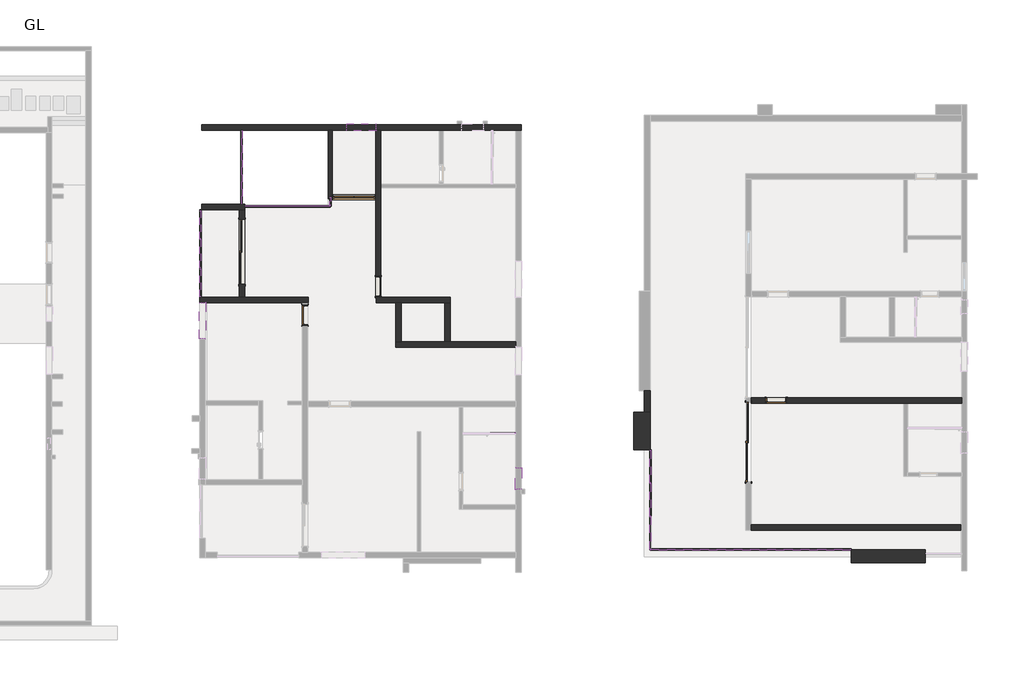
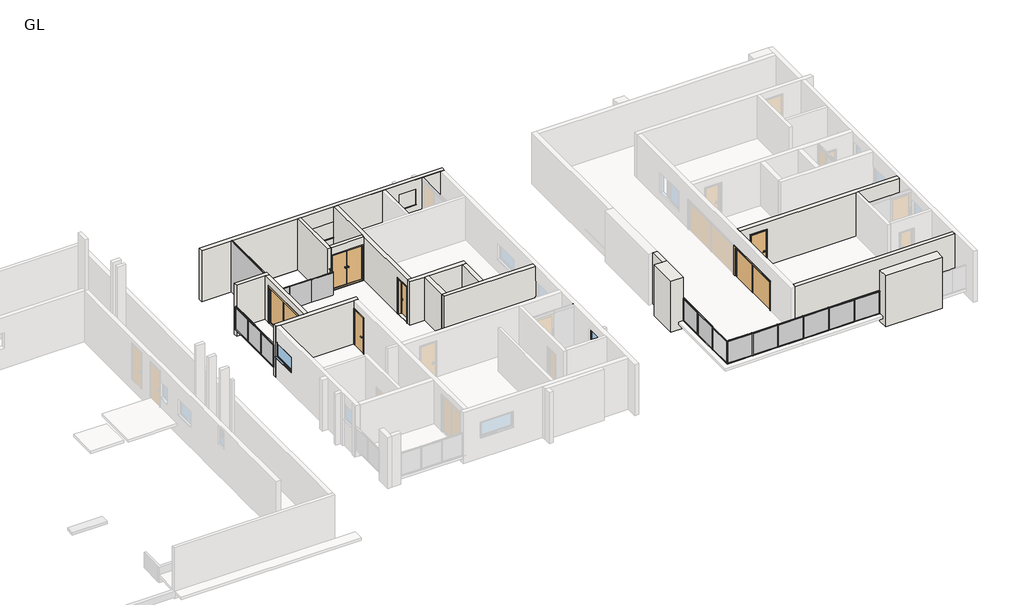
# One storey, part 3 of 6: 60 members, 17 walls, 16 plates, 6 doors, 3 windows.
# Revit data of these elements (continued)
# Elements 4, 5, 6 (IfcDoor, "Doors_IntSgl : 2'11\"") (continued)
#   Materials on its faces: "Door - Architrave", "Door - Handle", "Door - Frame/Mullion (1)", "Door - Panel"
# Elements 7, 8, 9, 10, 11, 12, 13, 14, 15, 16, 17, 18, 19, 20, 21, 22, 23, 24, 25, 26, 27, 28, 29, 30, 31, 32, 33, 34, 35, 36, 37, 38, 39, 40, 41, 42, 43, 44, 45, 46, 47, 48, 49, 50, 51, 52, 53, 54, 55, 56, 57, 58, 59, 60, 61, 62, 63, 64, 65, 66 (IfcMember, "Rectangular Mullion : 30mm_Square")
#   Phase Created = New Construction
#   Materials on its faces: "Aluminium"
# Elements 67, 68, 69, 70, 71, 72, 73, 74, 75, 76, 77, 78, 79, 80, 81, 82 (IfcPlate, "System Panel : Glazed")
#   Phase Created = New Construction
#   Materials on its faces: "Glass"
# Element 83 (IfcWall, "1'10\"")
#   Top Offset = 0' - 0"
#   Base Offset = 0' - 0"
#   wall height = 9' - 10.11024"
#   Phase Created = New Construction
#   Base Constraint = GL
#   Top Constraint = FFL
#   Materials on its faces: "Brick, Common"
# Element 84 (IfcWall, "10\"")
#   Top Offset = 0' - 0"
#   Base Offset = 0' - 0"
#   wall height = 9' - 10.11024"
#   Phase Created = New Construction
#   Base Constraint = GL
#   Top Constraint = FFL
#   Materials on its faces: "Brick, Common"
# Element 85 (IfcWall, "2'3\"")
#   Top Offset = 0' - 0"
#   Base Offset = 0' - 0"
#   wall height = 9' - 10.11024"
#   Phase Created = New Construction
#   Base Constraint = GL
#   Top Constraint = FFL
#   Materials on its faces: "Brick, Common"
# Elements 86, 87 (IfcWall, "7\" WALL")
#   Top Offset = 0' - 0"
#   Base Offset = 0' - 0"
#   wall height = 9' - 10.11024"
#   Phase Created = New Construction
#   Base Constraint = GL
#   Top Constraint = FFL
#   Materials on its faces: "Brick, Common"
# Elements 88, 89, 90, 91, 92, 93, 94, 95, 96, 97, 98, 99 (IfcWall, "9\" INNER WALL")
#   Top Offset = 0' - 0"
#   Base Offset = 0' - 0"
#   wall height = 9' - 10.11024"
#   Phase Created = New Construction
#   Base Constraint = GL
#   Top Constraint = FFL
#   Materials on its faces: "Brick, Common"
# Element 100 (IfcWindow, "Windows_Sgl_Plain : 3'")
#   Mark = "15"
#   Phase Created = New Construction
#   Materials on its faces: "Window Frame", "Glass"
# Element 101 (IfcWindow, "Windows_Sgl_Plain : 4'")
#   Mark = "11"
#   Phase Created = New Construction
#   Materials on its faces: "Window Frame", "Glass"
# Element 102 (IfcWindow, "Windows_Sgl_Plain : 5'")
#   Mark = "18"
#   Phase Created = New Construction
#   Materials on its faces: "Window Frame", "Glass"
# Materials
#   "Puerta - Panel": class "Madera", colour RGB 210 159 95, transparency 0
#   "Door - Panel": class "Wood", colour RGB 210 159 95, transparency 0, Keynote = "L20", Cost = 0
#   "Door - Frame/Mullion": class "Wood", colour RGB 212 179 113, transparency 0, Keynote = "L20", Cost = 0
#   "Door - Handle": colour RGB 0 0 0, transparency 0, Keynote = "P21", Cost = 0
#   "Door - Frame/Mullion (1)": class "Wood", colour RGB 212 179 113, transparency 0, Keynote = "L20", Cost = 0
#   "Door - Architrave": class "Wood", colour RGB 154 90 5, transparency 0, Keynote = "P20", Cost = 0
#   "Brick, Common": class "Masonry", colour RGB 170 100 105, transparency 0, Description = "Common brick", Cost = 0
#   "Window Frame": colour RGB 249 249 249, transparency 0, Keynote = "L10", Cost = 0
#   "Glass": class "Glass", colour RGB 0 128 192, transparency 0.9, Description = "Soda Lime Glass", Cost = 0
#   "Cristal": class "Vidrio", colour RGB 0 0 255, transparency 0.75
#   "Aluminium": class "Metal", colour RGB 247 247 247, transparency 0, Description = "Aluminium 6061", Cost = 0
